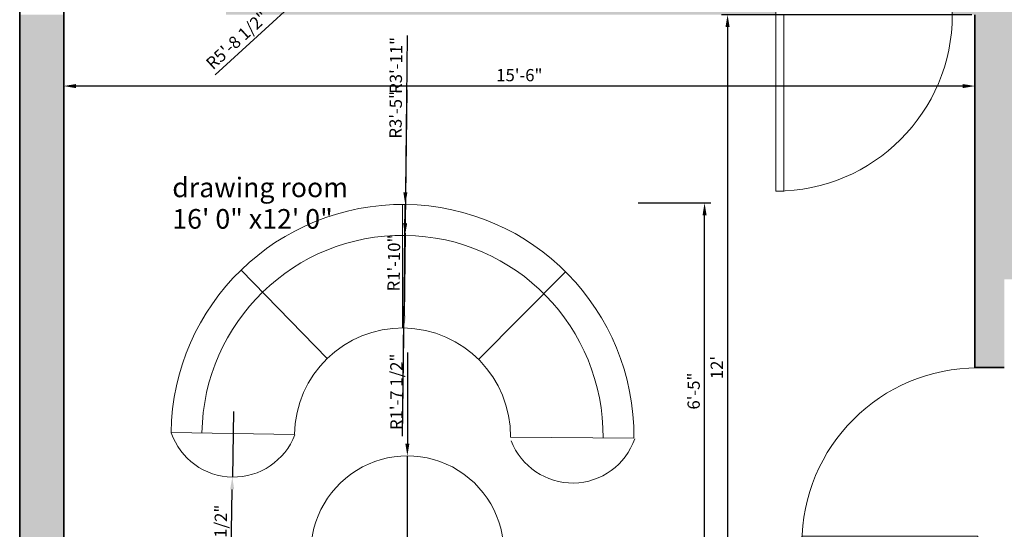
# Model space of a CAD drawing. Units: inches. Extents: x 2369 to 4208, y 1650 to 4492.
# Tile 2 of 6: x 2369 to 2570, y 1948 to 2052. Entities that reach past the tile are written whole.
import ezdxf

# ---------------------------------------------------------------- set-up
doc = ezdxf.new("R2010")
doc.units = ezdxf.units.IN
for name, color, linetype, lineweight in [('A-ANNO-DIMS', 2, 'Continuous', 13), ('A-AREA-IDEN', 7, 'Continuous', 18), ('A-DOOR', 4, 'Continuous', 18), ('A-FLOR-PATT', 9, 'Continuous', 13), ('A-FURN', 8, 'Continuous', 18), ('A-WALL', 7, 'Continuous', 35), ('A-WALL-PATT', 252, 'Continuous', 13)]:
    doc.layers.add(name, color=color, linetype=linetype, lineweight=lineweight)
doc.styles.get("Standard").update_dxf_attribs({"font": 'arial.ttf'})
doc.dimstyles.new('Copy of ISO-25', dxfattribs={"dimtxt": 2.5, "dimasz": 2.5, "dimexe": 1.25, "dimexo": 0.625, "dimtad": 1, "dimdec": 1, "dimlunit": 4, "dimtxsty": 'Standard', "dimcen": 2.5, "dimadec": 0, "dimazin": 0, "dimtfac": 1, "dimtdec": 1, "dimtmove": 0, "dimatfit": 3, "dimfxl": 1, "dimarcsym": 0})

# ---------------------------------------------------------------- blocks, each defined once
blk = doc.blocks.new('*U4')
for p, q in [((-40, 0), (-40, 6)), ((0, 0), (0, 6))]:
    blk.add_line(p, q)
blk.add_lwpolyline([(0, 0), (0, -40), (-1.75, -40), (-1.75, 0)], close=True)
blk.add_arc((0, 0), 40, 180, 270)
blk = doc.blocks.new('*U6')
for p, q in [((0, 0), (0, 6)), ((40, 0), (40, 6))]:
    blk.add_line(p, q)
blk.add_lwpolyline([(0, 0), (0, -40), (1.75, -40), (1.75, 0)], close=True)
blk.add_arc((0, 0), 40, 270, 0)
blk = doc.blocks.new('*D29')
at = {"layer": 'A-ANNO-DIMS', "color": 0, "lineweight": -2, "transparency": 16777216}
for p, q in [((2377.9, 2052.35), (2377.9, 2037.17)), ((2563.9, 2052.35), (2563.9, 2037.17)), ((2561.4, 2038.42), (2380.4, 2038.42))]:
    blk.add_line(p, q, dxfattribs=at)
at = {"layer": 'A-ANNO-DIMS', "color": 0, "transparency": 16777216}
for points in [[(2380.4, 2038.83), (2380.4, 2038), (2377.9, 2038.42)], [(2561.4, 2038.83), (2561.4, 2038), (2563.9, 2038.42)]]:
    blk.add_solid(points, dxfattribs=at)
at = {"layer": 'Defpoints', "color": 0, "transparency": 16777216}
for p in [(2377.9, 2052.98), (2563.9, 2052.98), (2377.9, 2038.42)]:
    blk.add_point(p, dxfattribs=at)
at = {"layer": 'A-ANNO-DIMS', "color": 0, "transparency": 16777216, "insert": (2470.9, 2040.32), "char_height": 2.5, "attachment_point": 5}
blk.add_mtext('15\'-6"', dxfattribs=at)
blk = doc.blocks.new('*D30')
at = {"layer": 'A-ANNO-DIMS', "color": 0, "lineweight": -2, "transparency": 16777216}
for p, q in [((2563.28, 2052.98), (2512.16, 2052.98)), ((2513.41, 2050.48), (2513.41, 1911.48)), ((2563.28, 1908.98), (2512.16, 1908.98))]:
    blk.add_line(p, q, dxfattribs=at)
at = {"layer": 'A-ANNO-DIMS', "color": 0, "transparency": 16777216}
for points in [[(2512.99, 2050.48), (2513.82, 2050.48), (2513.41, 2052.98)], [(2512.99, 1911.48), (2513.82, 1911.48), (2513.41, 1908.98)]]:
    blk.add_solid(points, dxfattribs=at)
at = {"layer": 'Defpoints', "color": 0, "transparency": 16777216}
for p in [(2563.9, 2052.98), (2513.41, 1908.98), (2563.9, 1908.98)]:
    blk.add_point(p, dxfattribs=at)
at = {"layer": 'A-ANNO-DIMS', "color": 0, "transparency": 16777216, "insert": (2511.53, 1980.98), "char_height": 2.5, "attachment_point": 5, "rotation": 90}
blk.add_mtext("12'", dxfattribs=at)
blk = doc.blocks.new('A$C22FC404C')
for p, q in [((1199.9, 1301.9), (1199.9, 1941.9)), ((809.2, 1143.1), (362.7, 1601.6)), ((1594.3, 1139.4), (2045.1, 1593.7)), ((0, 760.4), (639.9, 750.6)), ((2399.8, 731.4), (1759.8, 735.4)), ((827.3, 0), (1623.4, 0))]:
    blk.add_line(p, q)
for centre, radius, start, end in [((1199.9, 741.9), 1200, 359.499, 179.1174), ((1199.9, 741.9), 1040, 359.4096, 179.1174), ((1199.9, 741.9), 560, 359.3286, 179.1174), ((323.1, 869.6), 340.6, 199.1309, 339.1039), ((2082.3, 838.8), 340.6, 200.8961, 340.8691), ((1225.3, 139.3), 500, 354.3583, 185.6417), ((827.3, 100), 100, 185.6417, 270), ((1623.4, 100), 100, 270, 354.3583)]:
    blk.add_arc(centre, radius, start, end)
blk = doc.blocks.new('*D56')
at = {"layer": 'A-ANNO-DIMS', "color": 0, "lineweight": -2, "transparency": 16777216}
for p, q in [((2495.13, 2014.56), (2509.96, 2014.56)), ((2508.71, 1940.3), (2508.71, 2012.06)), ((2495.13, 1937.8), (2509.96, 1937.8))]:
    blk.add_line(p, q, dxfattribs=at)
at = {"layer": 'A-ANNO-DIMS', "color": 0, "transparency": 16777216}
for points in [[(2508.3, 2012.06), (2509.13, 2012.06), (2508.71, 2014.56)], [(2508.3, 1940.3), (2509.13, 1940.3), (2508.71, 1937.8)]]:
    blk.add_solid(points, dxfattribs=at)
at = {"layer": 'Defpoints', "color": 0, "transparency": 16777216}
for p in [(2494.51, 2014.56), (2508.71, 2014.56), (2494.51, 1937.8)]:
    blk.add_point(p, dxfattribs=at)
at = {"layer": 'A-ANNO-DIMS', "color": 0, "transparency": 16777216, "insert": (2506.81, 1976.18), "char_height": 2.5, "attachment_point": 5, "rotation": 90}
blk.add_mtext('6\'-5"', dxfattribs=at)
blk = doc.blocks.new('*D66')
at = {"layer": 'A-ANNO-DIMS', "color": 0, "lineweight": -2, "transparency": 16777216}
for p, q in [((2495.62, 2120.27), (2445.09, 2073.94)), ((2408.82, 2040.7), (2443.24, 2072.25))]:
    blk.add_line(p, q, dxfattribs=at)
at = {"layer": 'A-ANNO-DIMS', "color": 0, "transparency": 16777216}
blk.add_solid([(2442.96, 2072.56), (2443.52, 2071.94), (2445.09, 2073.94)], dxfattribs=at)
at = {"layer": 'Defpoints', "color": 0, "transparency": 16777216}
for p in [(2495.62, 2120.27), (2445.09, 2073.94)]:
    blk.add_point(p, dxfattribs=at)
at = {"layer": 'A-ANNO-DIMS', "color": 0, "transparency": 16777216, "insert": (2413.47, 2047.56), "char_height": 2.5, "attachment_point": 5, "rotation": 42.51}
blk.add_mtext('R5\'-8 1/2"', dxfattribs=at)
blk = doc.blocks.new('*D68')
at = {"layer": 'A-ANNO-DIMS', "color": 0, "lineweight": -2, "transparency": 16777216}
for p, q in [((2448.02, 2048.71), (2447.64, 2016.75)), ((2447.04, 1967.01), (2447.61, 2014.25))]:
    blk.add_line(p, q, dxfattribs=at)
at = {"layer": 'A-ANNO-DIMS', "color": 0, "transparency": 16777216}
blk.add_solid([(2447.22, 2016.75), (2448.05, 2016.74), (2447.61, 2014.25)], dxfattribs=at)
at = {"layer": 'Defpoints', "color": 0, "transparency": 16777216}
for p in [(2447.61, 2014.25), (2447.04, 1967.01)]:
    blk.add_point(p, dxfattribs=at)
at = {"layer": 'A-ANNO-DIMS', "color": 0, "transparency": 16777216, "insert": (2446.05, 2042.62), "char_height": 2.5, "attachment_point": 5, "rotation": 89.308}
blk.add_mtext('R3\'-11"', dxfattribs=at)
blk = doc.blocks.new('*D69')
at = {"layer": 'A-ANNO-DIMS', "color": 0, "lineweight": -2, "transparency": 16777216}
for p, q in [((2447.95, 2037.66), (2447.6, 2010.45)), ((2447.04, 1967.01), (2447.56, 2007.95))]:
    blk.add_line(p, q, dxfattribs=at)
at = {"layer": 'A-ANNO-DIMS', "color": 0, "transparency": 16777216}
blk.add_solid([(2447.18, 2010.45), (2448.01, 2010.44), (2447.56, 2007.95)], dxfattribs=at)
at = {"layer": 'Defpoints', "color": 0, "transparency": 16777216}
for p in [(2447.56, 2007.95), (2447.04, 1967.01)]:
    blk.add_point(p, dxfattribs=at)
at = {"layer": 'A-ANNO-DIMS', "color": 0, "transparency": 16777216, "insert": (2445.98, 2032.54), "char_height": 2.5, "attachment_point": 5, "rotation": 89.2632}
blk.add_mtext('R3\'-5"', dxfattribs=at)
blk = doc.blocks.new('*D70')
at = {"layer": 'A-ANNO-DIMS', "color": 0, "lineweight": -2, "transparency": 16777216}
for p, q in [((2447.6, 2008.4), (2447.37, 1991.55)), ((2447.04, 1967.01), (2447.34, 1989.05))]:
    blk.add_line(p, q, dxfattribs=at)
at = {"layer": 'A-ANNO-DIMS', "color": 0, "transparency": 16777216}
blk.add_solid([(2446.95, 1991.56), (2447.79, 1991.55), (2447.34, 1989.05)], dxfattribs=at)
at = {"layer": 'Defpoints', "color": 0, "transparency": 16777216}
for p in [(2447.34, 1989.05), (2447.04, 1967.01)]:
    blk.add_point(p, dxfattribs=at)
at = {"layer": 'A-ANNO-DIMS', "color": 0, "transparency": 16777216, "insert": (2445.61, 2002.31), "char_height": 2.5, "attachment_point": 5, "rotation": 89.2241}
blk.add_mtext('R1\'-10"', dxfattribs=at)
blk = doc.blocks.new('*D71')
at = {"layer": 'A-ANNO-DIMS', "color": 0, "lineweight": -2, "transparency": 16777216}
for p, q in [((2448.04, 1984.08), (2448.04, 1965.47)), ((2448.04, 1943.28), (2448.04, 1962.97))]:
    blk.add_line(p, q, dxfattribs=at)
at = {"layer": 'A-ANNO-DIMS', "color": 0, "transparency": 16777216}
blk.add_solid([(2447.62, 1965.47), (2448.46, 1965.47), (2448.04, 1962.97)], dxfattribs=at)
at = {"layer": 'Defpoints', "color": 0, "transparency": 16777216}
for p in [(2448.04, 1962.97), (2448.04, 1943.28)]:
    blk.add_point(p, dxfattribs=at)
at = {"layer": 'A-ANNO-DIMS', "color": 0, "transparency": 16777216, "insert": (2446.12, 1976.03), "char_height": 2.5, "attachment_point": 5, "rotation": 89.9986}
blk.add_mtext('R1\'-7 1/2"', dxfattribs=at)
blk = doc.blocks.new('*D72')
at = {"layer": 'A-ANNO-DIMS', "color": 0, "lineweight": -2, "transparency": 16777216}
for p, q in [((2412.52, 1972.03), (2412.31, 1958.63)), ((2411.91, 1932.1), (2412.28, 1956.13))]:
    blk.add_line(p, q, dxfattribs=at)
at = {"layer": 'A-ANNO-DIMS', "color": 0, "transparency": 16777216}
blk.add_solid([(2411.86, 1956.13), (2412.69, 1956.12), (2412.31, 1958.63)], dxfattribs=at)
at = {"layer": 'Defpoints', "color": 0, "transparency": 16777216}
for p in [(2412.52, 1972.03), (2412.31, 1958.63)]:
    blk.add_point(p, dxfattribs=at)
at = {"layer": 'A-ANNO-DIMS', "color": 0, "transparency": 16777216, "insert": (2410.16, 1942.89), "char_height": 2.5, "attachment_point": 5, "rotation": 89.1191}
blk.add_mtext('2X R1\'-1 1/2"', dxfattribs=at)

msp = doc.modelspace()

# ---------------------------------------------------------------- hatches: boundary and pattern name
at = {"layer": 'A-FLOR-PATT'}
h = msp.add_hatch(dxfattribs=at)
h.set_pattern_fill('ANGLE', color=256)
h.set_pattern_definition([(0, (0, 0), (0, 6.985), [5.08, -1.905]), (90, (0, 0), (-6.985, 4e-16), [5.08, -1.905])])
h.paths.add_polyline_path([(2599.9, 2460.98), (2551.9, 2460.98), (2551.9, 2298.98), (2563.9, 2298.98), (2563.9, 2306.63), (2564.42, 2306.63), (2564.42, 2306.61, -0.405418), (2575.94, 2294.77, -0.401619), (2587.38, 2306.72), (2587.38, 2306.73), (2587.9, 2306.73), (2587.9, 2298.98), (2599.9, 2298.98)])
h.paths.add_polyline_path([(2425.9, 2226.98), (2377.9, 2226.98), (2377.9, 2154.98), (2389.9, 2154.98), (2425.9, 2154.98)])
h.paths.add_polyline_path([(2641.9, 2052.98), (2569.9, 2052.98), (2569.9, 1998.98), (2581.9, 1998.98), (2581.9, 1992.98), (2606.44, 1992.98), (2629.9, 1992.98), (2629.9, 1998.98), (2641.9, 1998.98), (2641.9, 2008.36), (2647.9, 2008.36), (2647.9, 1956.98), (2767.9, 1956.98), (2767.9, 2052.98), (2647.9, 2052.98), (2647.9, 2044.36), (2641.9, 2044.36)])
h.paths.add_polyline_path([(2628.69, 2019.73), (2629.71, 2019.73), (2629.71, 1996.47), (2628.69, 1996.47)], flags=16)
h.paths.add_polyline_path([(2563.51, 2406.86), (2576.05, 2406.86), (2576.05, 2412.82), (2563.51, 2412.82)], flags=24)
h.paths.add_polyline_path([(2391.33, 2190.25), (2403.87, 2190.25), (2403.87, 2196.21), (2391.33, 2196.21)], flags=24)
h.paths.add_polyline_path([(2704.89, 2039.23), (2710.69, 2039.23), (2710.69, 2044.38), (2704.89, 2044.38)], flags=24)
h.paths.add_polyline_path([(2759.77, 2003.06), (2759.77, 2006.92), (2754.62, 2006.92), (2754.62, 2003.06)], flags=24)
h.paths.add_polyline_path([(2707.15, 2003.75), (2738.28, 2003.75), (2738.28, 2009.88), (2707.15, 2009.88)], flags=24)
h.paths.add_polyline_path([(2707.15, 2010.19), (2726.89, 2010.19), (2726.89, 2016.29), (2707.15, 2016.29)], flags=24)
h.paths.add_polyline_path([(2577.31, 2031), (2605.34, 2031), (2605.34, 2037.12), (2577.31, 2037.12)], flags=24)
h.paths.add_polyline_path([(2577.02, 2036.02), (2603.33, 2036.02), (2603.33, 2043.89), (2577.02, 2043.89)], flags=24)
at = {"layer": 'A-WALL-PATT'}
h = msp.add_hatch(color=256, dxfattribs=at)
h.dxf.hatch_style = 1
h.paths.add_polyline_path([(2377.9, 2052.98), (2368.9, 2052.98), (2368.9, 1926.53), (2377.9, 1926.53)])
h.paths.add_polyline_path([(2377.9, 2226.98), (2368.9, 2226.98), (2368.9, 2079.34), (2377.9, 2079.34)])
h.paths.add_polyline_path([(2377.9, 2394.98), (2377.9, 2460.98), (2767.9, 2460.98), (2767.9, 2250.53), (2776.9, 2250.53), (2776.9, 2469.98), (2368.9, 2469.98), (2368.9, 2254.21), (2377.9, 2254.21)])
h.paths.add_polyline_path([(2776.9, 2226.98), (2767.9, 2226.98), (2767.9, 2078.3), (2776.9, 2078.3)])
h.paths.add_polyline_path([(2776.9, 2052.98), (2767.9, 2052.98), (2767.9, 1973.96), (2776.9, 1973.96)])
h.paths.add_polyline_path([(2776.9, 1950.98), (2767.9, 1950.98), (2767.9, 1775.33), (2776.9, 1775.33)])
h.paths.add_polyline_path([(2560.9, 1758.98), (2377.9, 1758.98), (2377.9, 1749.98), (2386.24, 1749.98), (2386.07, 1750.89), (2387.22, 1749.98), (2560.9, 1749.98)])
h.paths.add_polyline_path([(2377.9, 1902.98), (2368.9, 1902.98), (2368.9, 1774.03), (2377.9, 1774.03)])
h.paths.add_polyline_path([(2569.9, 1908.98), (2569.9, 1944.98), (2563.9, 1944.98), (2563.9, 1908.98), (2377.9, 1908.98), (2377.9, 1902.98), (2569.9, 1902.98)])
h.paths.add_polyline_path([(2523.29, 2058.98), (2411, 2058.98), (2411, 2052.98), (2523.29, 2052.98)])
h.paths.add_polyline_path([(2569.9, 2052.98), (2641.9, 2052.98), (2713.81, 2052.98), (2713.81, 2058.98), (2559.29, 2058.98), (2559.29, 2052.98), (2563.9, 2052.98), (2563.9, 1980.98), (2569.9, 1980.98), (2569.9, 1992.98)])
h.paths.add_polyline_path([(2528.53, 2232.98), (2510.56, 2232.98), (2377.9, 2232.98), (2377.9, 2226.98), (2528.53, 2226.98)])
h.paths.add_polyline_path([(2713.81, 2232.98), (2623.27, 2232.98), (2623.27, 2226.98), (2713.81, 2226.98)])
h.paths.add_polyline_path([(2647.9, 2008.36), (2642.51, 2008.36), (2641.9, 2008.36), (2641.9, 1956.98), (2641.9, 1950.98), (2767.9, 1950.98), (2767.9, 1956.98), (2647.9, 1956.98)])
h.paths.add_polyline_path([(2551.9, 2395.12), (2545.9, 2395.12), (2545.9, 2268.98), (2551.9, 2268.98)], flags=17)
h.paths.add_polyline_path([(2551.9, 2460.98), (2545.9, 2460.98), (2545.9, 2400.98), (2551.9, 2400.98)], flags=17)
h.paths.add_polyline_path([(2605.9, 2460.98), (2599.9, 2460.98), (2599.9, 2400.98), (2605.9, 2400.98)], flags=17)
h.paths.add_polyline_path([(2767.9, 2400.98), (2637.99, 2400.98), (2637.99, 2394.98), (2767.9, 2394.98)], flags=17)
h.paths.add_polyline_path([(2605.9, 2394.98), (2599.9, 2394.98), (2599.9, 2394.42), (2599.9, 2268.98), (2605.9, 2268.98)], flags=17)
h.paths.add_polyline_path([(2525.15, 2400.98), (2377.9, 2400.98), (2377.9, 2394.98), (2525.15, 2394.98)], flags=17)
h.paths.add_polyline_path([(2449.9, 2412.98), (2444.51, 2412.98), (2443.9, 2412.98), (2443.9, 2400.98), (2449.9, 2400.98)], flags=17)
h.paths.add_polyline_path([(2449.9, 2460.98), (2443.9, 2460.98), (2443.9, 2448.98), (2449.9, 2448.98)], flags=17)
h.paths.add_polyline_path([(2731.9, 2106.98), (2725.9, 2106.98), (2725.9, 2058.98), (2731.9, 2058.98)])

# ---------------------------------------------------------------- linework, layer by layer
at = {"layer": 'A-WALL'}
for p, q in [((2377.9, 2052.98), (2377.9, 1908.98)), ((2563.9, 1980.98), (2563.9, 2052.98)), ((2569.9, 1980.98), (2563.9, 1980.98))]:
    msp.add_line(p, q, dxfattribs=at)
for points in [[(2368.9, 1749.98), (2368.9, 2469.98), (2776.9, 2469.98), (2776.9, 1749.98), (2689.9, 1749.98)], [(2767.9, 2052.98), (2767.9, 1758.98), (2377.9, 1758.98), (2377.9, 2460.98), (2767.9, 2460.98), (2767.9, 2232.98)]]:
    msp.add_lwpolyline(points, dxfattribs=at)

# ---------------------------------------------------------------- block references
at = {"layer": 'A-DOOR', "xscale": 0.8998204407006335, "yscale": 0.8998204407006335, "zscale": 0.8998204407006335}
msp.add_blockref('*U6', (2523.29, 2052.98), dxfattribs=at)
at = {"layer": 'A-DOOR', "xscale": 0.8987594980764617, "yscale": 0.8987594980764617, "zscale": 0.8987594980764617, "rotation": 270}
msp.add_blockref('*U4', (2564.51, 1944.98), dxfattribs=at)
at = {"layer": 'A-FURN', "xscale": 0.0393700787401575, "yscale": 0.0393700787401575, "zscale": 0.0393700787401575}
msp.add_blockref('A$C22FC404C', (2399.8, 1937.8), dxfattribs=at)

# ---------------------------------------------------------------- texts
at = {"layer": 'A-AREA-IDEN'}
for s, p in [('drawing room', (2400.05, 2015.74)), ('16\' 0" x12\' 0"', (2400.05, 2009.32))]:
    msp.add_text(s, height=4, dxfattribs=at).set_placement(p)

# ---------------------------------------------------------------- dimensions: what is measured, and where the dimension line sits
at = {"layer": 'A-ANNO-DIMS'}
for center, mpoint, picture, middle in [((2495.62, 2120.27), (2445.09, 2073.94), '*D66', (2414.76, 2046.14)), ((2447.04, 1967.01), (2447.61, 2014.25), '*D68', (2447.95, 2042.59)), ((2447.04, 1967.01), (2447.56, 2007.95), '*D69', (2447.88, 2032.51)), ((2447.04, 1967.01), (2447.34, 1989.05), '*D70', (2447.52, 2002.28))]:
    dim = msp.add_radius_dim(center=center, mpoint=mpoint, dimstyle='Copy of ISO-25', override={"dimdec": 1, "dimlfac": 1, "dimrnd": 0, "dimzin": 1, "dimdsep": 46, "dimlunit": 4, "dimfrac": 2}, dxfattribs=at)
    dim.commit()
    dim.dimension.update_dxf_attribs({"geometry": picture, "text_midpoint": middle, "dimtype": 164})
dim = msp.add_linear_dim(base=(2377.9, 2038.42), p1=(2563.9, 2052.98), p2=(2377.9, 2052.98), dimstyle='Copy of ISO-25', override={"dimclrd": 0, "dimclre": 0, "dimclrt": 0}, dxfattribs=at)
dim.commit()
dim.dimension.update_dxf_attribs({"geometry": '*D29', "text_midpoint": (2470.9, 2040.32)})
for base, p1, p2, override, picture, middle in [((2513.41, 1908.98), (2563.9, 2052.98), (2563.9, 1908.98), {"dimclrd": 0, "dimclre": 0, "dimclrt": 0}, '*D30', (2511.53, 1980.98)), ((2508.71, 2014.56), (2494.51, 1937.8), (2494.51, 2014.56), {"dimdec": 1, "dimlfac": 1, "dimrnd": 0, "dimzin": 1, "dimdsep": 46, "dimlunit": 4, "dimfrac": 2}, '*D56', (2506.81, 1976.18))]:
    dim = msp.add_linear_dim(base=base, p1=p1, p2=p2, angle=90, dimstyle='Copy of ISO-25', override=override, dxfattribs=at)
    dim.commit()
    dim.dimension.update_dxf_attribs({"geometry": picture, "text_midpoint": middle})
dim = msp.add_radius_dim(center=(2448.04, 1943.28), mpoint=(2448.04, 1962.97), dimstyle='Copy of ISO-25', override={"dimdec": 1, "dimlfac": 1, "dimrnd": 0, "dimzin": 1, "dimdsep": 46, "dimlunit": 4, "dimfrac": 2}, dxfattribs=at)
dim.commit()
dim.dimension.update_dxf_attribs({"geometry": '*D71', "text_midpoint": (2446.12, 1976.03)})
dim = msp.add_radius_dim(center=(2412.52, 1972.03), mpoint=(2412.31, 1958.63), text='2X <>', dimstyle='Copy of ISO-25', override={"dimdec": 1, "dimlfac": 1, "dimrnd": 0, "dimzin": 1, "dimdsep": 46, "dimlunit": 4, "dimfrac": 2}, dxfattribs=at)
dim.commit()
dim.dimension.update_dxf_attribs({"geometry": '*D72', "text_midpoint": (2410.16, 1942.89)})

doc.saveas('drawing.dxf')
